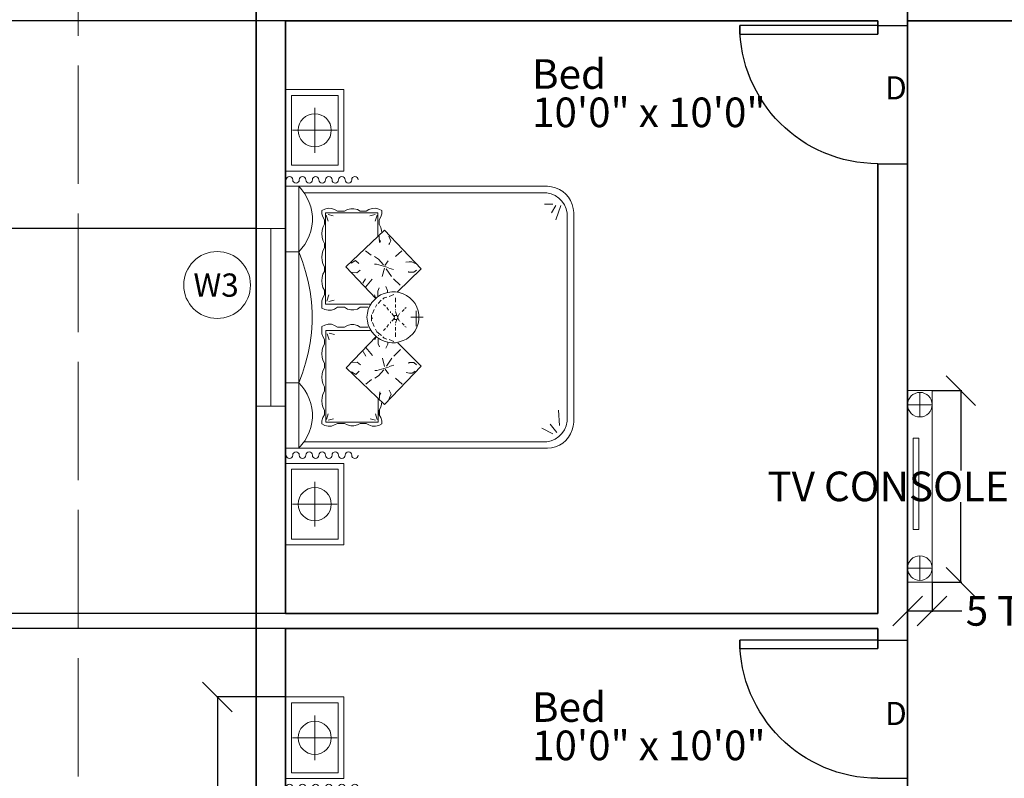
# Model space of a CAD drawing. Units: inches. Extents: x -1198 to -69, y -512 to 437.
# Tile 4 of 50: x -1067 to -867, y 5 to 158. Entities that reach past the tile are written whole.
import ezdxf

# ---------------------------------------------------------------- set-up
doc = ezdxf.new("R2010")
doc.units = ezdxf.units.IN
doc.header["$MEASUREMENT"] = 0
doc.linetypes.add('ACAD_ISO02W100', pattern=[15, 12, -3])
for name, color, linetype, lineweight in [('A-ANNO-DIMS', 2, 'Continuous', 18), ('A-ANNO-SYMB', 7, 'Continuous', 18), ('A-AREA-IDEN', 7, 'Continuous', 18), ('A-EQPM', 60, 'Continuous', 18), ('A-FURN', 60, 'Continuous', 18), ('A-WALL', 7, 'Continuous', 35), ('C-PROP', 141, 'ACAD_ISO02W100', 18), ('Doors', 140, 'Continuous', 25), ('ds_furniture_Pen_No__7', 7, 'Continuous', 18), ('windows', 160, 'Continuous', 18)]:
    doc.layers.add(name, color=color, linetype=linetype, lineweight=lineweight)
doc.styles.get("Standard").update_dxf_attribs({"font": 'arial.ttf'})
doc.dimstyles.get("Standard").update_dxf_attribs({"dimtxt": 6, "dimasz": 6, "dimexe": 0.18, "dimexo": 0.0625, "dimgap": 0.09, "dimtad": 0, "dimtih": 1, "dimtoh": 1, "dimdec": 0, "dimzin": 0, "dimdsep": 46, "dimlunit": 4, "dimtxsty": 'Standard', "dimblk": 'OBLIQUE', "dimcen": 0.09, "dimadec": 0, "dimazin": 0, "dimtfac": 1, "dimtdec": 0, "dimtofl": 0, "dimtmove": 0, "dimatfit": 3, "dimfxl": 1, "dimtolj": 1, "dimtzin": 0, "dimarcsym": 0})

# ---------------------------------------------------------------- blocks, each defined once
blk = doc.blocks.new('*U4')
for p, q in [((0, 0), (0, -6)), ((28, 0), (28, -6))]:
    blk.add_line(p, q)
blk.add_lwpolyline([(0, 0), (0, 28), (1.75, 28), (1.75, 0)], close=True)
blk.add_arc((0, 0), 28, 0, 90)
blk = doc.blocks.new('new')
at = {"layer": 'ds_furniture_Pen_No__7'}
for p, q in [((-1180, 2274.4), (-1838.2, 2274.4)), ((-1838.2, 2274.4), (-1838.2, 1804.2)), ((-1227, 2227.4), (-1791.2, 2227.4)), ((-1791.2, 2227.4), (-1791.2, 1851.2)), ((-1227, 1851.2), (-1227, 2227.4)), ((-1180, 1804.2), (-1180, 2274.4)), ((-1057.8, 158.7), (-1057.8, 2274.4)), ((-1057.8, 2274.4), (1057.8, 2274.4)), ((-1057.8, 2274.4), (1057.8, 2274.4)), ((-1057.8, 158.7), (-1057.8, 2274.4)), ((-528.9, 2274.4), (-528.9, 2168.6)), ((528.9, 2274.4), (528.9, 2168.6)), ((1057.8, 2274.4), (1057.8, 158.7)), ((1057.8, 2274.4), (1057.8, 158.7)), ((1180, 1804.2), (1180, 2274.4)), ((1180, 2274.4), (1838.2, 2274.4)), ((1227, 1851.2), (1227, 2227.4)), ((1227, 2227.4), (1791.2, 2227.4)), ((1791.2, 2227.4), (1791.2, 1851.2)), ((1838.2, 2274.4), (1838.2, 1804.2)), ((-1509.1, 2220.2), (-1509.1, 1858.4)), ((1057.8, 2168.6), (-1057.8, 2168.6)), ((-1057.8, 2168.6), (-1028.2, 2143.2)), ((-556.4, 2143.2), (-528.9, 2168.6)), ((-528.9, 2168.6), (-450.6, 2139)), ((450.6, 2139), (528.9, 2168.6)), ((528.9, 2168.6), (556.4, 2143.2)), ((1028.2, 2143.2), (1057.8, 2168.6)), ((1509.1, 2220.2), (1509.1, 1858.4)), ((-1028.2, 2143.2), (-996.5, 2119.9)), ((-1005, 165), (-1005, 2124.2)), ((-996.5, 2119.9), (-962.6, 2100.9)), ((-962.6, 2100.9), (-926.7, 2084)), ((-926.7, 2084), (-890.7, 2071.3)), ((-890.7, 2071.3), (-850.5, 2062.8)), ((-734.1, 2062.8), (-696.1, 2071.3)), ((-696.1, 2071.3), (-658, 2084)), ((-658, 2084), (-622, 2100.9)), ((-622, 2100.9), (-588.2, 2119.9)), ((-588.2, 2119.9), (-556.4, 2143.2)), ((-450.6, 2139), (-370.2, 2113.6)), ((-370.2, 2113.6), (-289.9, 2092.4)), ((-289.9, 2092.4), (-207.3, 2075.5)), ((-207.3, 2075.5), (-124.8, 2064.9)), ((124.8, 2064.9), (207.3, 2075.5)), ((207.3, 2075.5), (289.9, 2092.4)), ((289.9, 2092.4), (370.2, 2113.6)), ((370.2, 2113.6), (450.6, 2139)), ((556.4, 2143.2), (588.2, 2119.9)), ((588.2, 2119.9), (622, 2100.9)), ((622, 2100.9), (658, 2084)), ((658, 2084), (696.1, 2071.3)), ((696.1, 2071.3), (734.1, 2062.8)), ((850.5, 2062.8), (890.7, 2071.3)), ((890.7, 2071.3), (926.7, 2084)), ((926.7, 2084), (962.6, 2100.9)), ((962.6, 2100.9), (996.5, 2119.9)), ((996.5, 2119.9), (1028.2, 2143.2)), ((1005, 2124.2), (1005, 165)), ((-1690.1, 2039.3), (-1328.2, 2039.3)), ((-850.5, 2062.8), (-812.4, 2058.6)), ((-812.4, 2058.6), (-772.2, 2058.6)), ((-772.2, 2058.6), (-734.1, 2062.8)), ((-124.8, 2064.9), (-42.3, 2060.7)), ((-42.3, 2060.7), (42.3, 2060.7)), ((42.3, 2060.7), (124.8, 2064.9)), ((734.1, 2062.8), (772.2, 2058.6)), ((772.2, 2058.6), (812.4, 2058.6)), ((812.4, 2058.6), (850.5, 2062.8)), ((1690.1, 2039.3), (1328.2, 2039.3)), ((-880.1, 1931.6), (-873.8, 1959.1)), ((-878, 1904.1), (-880.1, 1931.6)), ((-873.8, 1959.1), (-861.1, 1982.4)), ((-861.1, 1982.4), (-835.7, 1982.4)), ((-846.3, 1527.5), (-846.3, 1950.7)), ((-846.3, 1950.7), (-107.9, 1950.7)), ((-835.7, 1982.4), (-810.3, 1973.9)), ((-831.5, 1929.5), (-820.9, 1887.2)), ((-825.1, 1944.3), (-778.6, 1929.5)), ((-810.3, 1973.9), (-787, 1961.2)), ((-787, 1961.2), (-751.1, 1961.2)), ((-751.1, 1961.2), (-725.7, 1973.9)), ((-725.7, 1973.9), (-700.3, 1980.3)), ((-700.3, 1980.3), (-674.9, 1982.4)), ((-674.9, 1982.4), (-647.4, 1980.3)), ((-647.4, 1980.3), (-622, 1973.9)), ((-622, 1973.9), (-596.6, 1961.2)), ((-596.6, 1961.2), (-560.7, 1961.2)), ((-560.7, 1961.2), (-535.3, 1973.9)), ((-535.3, 1973.9), (-509.9, 1980.3)), ((-509.9, 1980.3), (-484.5, 1982.4)), ((-484.5, 1982.4), (-457, 1980.3)), ((-457, 1980.3), (-431.6, 1973.9)), ((-431.6, 1973.9), (-408.3, 1961.2)), ((-408.3, 1961.2), (-370.2, 1961.2)), ((-370.2, 1961.2), (-347, 1973.9)), ((-347, 1973.9), (-321.6, 1980.3)), ((-321.6, 1980.3), (-294.1, 1982.4)), ((-294.1, 1982.4), (-266.6, 1980.3)), ((-266.6, 1980.3), (-241.2, 1973.9)), ((-241.2, 1973.9), (-217.9, 1961.2)), ((-217.9, 1961.2), (-179.8, 1961.2)), ((-133.3, 1940.1), (-181.9, 1923.2)), ((-179.8, 1961.2), (-156.6, 1973.9)), ((-156.6, 1973.9), (-133.3, 1982.4)), ((-129.1, 1923.2), (-139.6, 1880.9)), ((-133.3, 1982.4), (-105.8, 1982.4)), ((-107.9, 1950.7), (-107.9, 1591)), ((-105.8, 1982.4), (-74, 1982.4)), ((-74, 1982.4), (-63.5, 1959.1)), ((-63.5, 1959.1), (-57.1, 1931.6)), ((-57.1, 1931.6), (-57.1, 1904.1)), ((63.5, 1959.1), (57.1, 1931.6)), ((57.1, 1931.6), (57.1, 1904.1)), ((74, 1982.4), (63.5, 1959.1)), ((105.8, 1982.4), (74, 1982.4)), ((133.3, 1982.4), (105.8, 1982.4)), ((844.2, 1952.8), (105.8, 1952.8)), ((105.8, 1952.8), (105.8, 1593.1)), ((126.9, 1925.3), (137.5, 1883)), ((131.2, 1942.2), (179.8, 1925.3)), ((156.6, 1973.9), (133.3, 1982.4)), ((179.8, 1961.2), (156.6, 1973.9)), ((217.9, 1961.2), (179.8, 1961.2)), ((241.2, 1973.9), (217.9, 1961.2)), ((266.6, 1980.3), (241.2, 1973.9)), ((294.1, 1982.4), (266.6, 1980.3)), ((321.6, 1980.3), (294.1, 1982.4)), ((347, 1973.9), (321.6, 1980.3)), ((370.2, 1961.2), (347, 1973.9)), ((408.3, 1961.2), (370.2, 1961.2)), ((431.6, 1973.9), (408.3, 1961.2)), ((457, 1980.3), (431.6, 1973.9)), ((484.5, 1982.4), (457, 1980.3)), ((509.9, 1980.3), (484.5, 1982.4)), ((535.3, 1973.9), (509.9, 1980.3)), ((560.7, 1961.2), (535.3, 1973.9)), ((596.6, 1961.2), (560.7, 1961.2)), ((622, 1973.9), (596.6, 1961.2)), ((647.4, 1980.3), (622, 1973.9)), ((674.9, 1982.4), (647.4, 1980.3)), ((700.3, 1980.3), (674.9, 1982.4)), ((725.7, 1973.9), (700.3, 1980.3)), ((751.1, 1961.2), (725.7, 1973.9)), ((787, 1961.2), (751.1, 1961.2)), ((823, 1946.4), (776.5, 1931.6)), ((810.3, 1973.9), (787, 1961.2)), ((835.7, 1982.4), (810.3, 1973.9)), ((829.4, 1931.6), (818.8, 1889.3)), ((861.1, 1982.4), (835.7, 1982.4)), ((844.2, 1529.6), (844.2, 1952.8)), ((873.8, 1959.1), (861.1, 1982.4)), ((880.1, 1931.6), (873.8, 1959.1)), ((878, 1904.1), (880.1, 1931.6)), ((-1791.2, 1851.2), (-1227, 1851.2)), ((-869.6, 1878.7), (-878, 1904.1)), ((-856.9, 1855.5), (-869.6, 1878.7)), ((-856.9, 1798.3), (-856.9, 1855.5)), ((-65.6, 1878.7), (-80.4, 1855.5)), ((-80.4, 1855.5), (-80.4, 1798.3)), ((-57.1, 1904.1), (-65.6, 1878.7)), ((57.1, 1904.1), (65.6, 1878.7)), ((65.6, 1878.7), (80.4, 1855.5)), ((80.4, 1855.5), (80.4, 1798.3)), ((856.9, 1855.5), (869.6, 1878.7)), ((856.9, 1798.3), (856.9, 1855.5)), ((869.6, 1878.7), (878, 1904.1)), ((1791.2, 1851.2), (1227, 1851.2)), ((-1838.2, 1804.2), (-1180, 1804.2)), ((-875.9, 1747.6), (-869.6, 1775.1)), ((-869.6, 1775.1), (-856.9, 1798.3)), ((-704.5, 1474.6), (-408.3, 1785.6)), ((-408.3, 1785.6), (-154.4, 1544.5)), ((-366, 1749.7), (-361.8, 1696.8)), ((-80.4, 1798.3), (-65.6, 1775.1)), ((-65.6, 1775.1), (-59.2, 1747.6)), ((65.6, 1775.1), (59.2, 1747.6)), ((80.4, 1798.3), (65.6, 1775.1)), ((406.2, 1787.8), (152.3, 1546.6)), ((363.9, 1751.8), (359.7, 1698.9)), ((702.4, 1476.8), (406.2, 1787.8)), ((869.6, 1775.1), (856.9, 1798.3)), ((875.9, 1747.6), (869.6, 1775.1)), ((1838.2, 1804.2), (1180, 1804.2)), ((-875.9, 1722.2), (-875.9, 1747.6)), ((-869.6, 1694.7), (-875.9, 1722.2)), ((-856.9, 1671.4), (-869.6, 1694.7)), ((-856.9, 1624.9), (-856.9, 1671.4)), ((-440.1, 1743.3), (-461.2, 1707.4)), ((-461.2, 1707.4), (-435.8, 1679.9)), ((-361.8, 1696.8), (-382.9, 1669.3)), ((-65.6, 1694.7), (-80.4, 1671.4)), ((-80.4, 1671.4), (-80.4, 1607.9)), ((-59.2, 1722.2), (-65.6, 1694.7)), ((-59.2, 1747.6), (-59.2, 1722.2)), ((59.2, 1747.6), (59.2, 1722.2)), ((59.2, 1722.2), (65.6, 1694.7)), ((65.6, 1694.7), (80.4, 1671.4)), ((80.4, 1671.4), (80.4, 1607.9)), ((359.7, 1698.9), (380.8, 1671.4)), ((459.1, 1709.5), (433.7, 1682)), ((437.9, 1745.4), (459.1, 1709.5)), ((856.9, 1671.4), (869.6, 1694.7)), ((856.9, 1624.9), (856.9, 1671.4)), ((869.6, 1694.7), (875.9, 1722.2)), ((875.9, 1722.2), (875.9, 1747.6)), ((-878, 1576.2), (-869.6, 1601.6)), ((-869.6, 1601.6), (-856.9, 1624.9)), ((-831.5, 1548.7), (-820.9, 1591)), ((-539.5, 1627), (-503.5, 1580.4)), ((-277.2, 1648.1), (-313.1, 1627)), ((-245.4, 1627), (-308.9, 1574.1)), ((-118.5, 1578.3), (-91, 1595.2)), ((-91, 1595.2), (-61.4, 1607.9)), ((-61.4, 1607.9), (-31.7, 1614.3)), ((-31.7, 1614.3), (0, 1618.5)), ((0, 1618.5), (31.7, 1614.3)), ((31.7, 1614.3), (61.4, 1607.9)), ((61.4, 1607.9), (91, 1595.2)), ((91, 1595.2), (118.5, 1578.3)), ((243.3, 1629.1), (306.8, 1576.2)), ((275, 1650.2), (311, 1629.1)), ((537.4, 1629.1), (501.4, 1582.5)), ((829.4, 1550.8), (818.8, 1593.1)), ((869.6, 1601.6), (856.9, 1624.9)), ((878, 1576.2), (869.6, 1601.6)), ((-880.1, 1548.7), (-878, 1576.2)), ((-873.8, 1521.2), (-880.1, 1548.7)), ((-861.1, 1497.9), (-873.8, 1521.2)), ((-651.6, 1527.5), (-846.3, 1527.5)), ((-825.1, 1533.9), (-778.6, 1548.7)), ((-787, 1519.1), (-810.3, 1506.4)), ((-772.2, 1517), (-789.2, 1517)), ((-751.1, 1519.1), (-787, 1519.1)), ((-761.7, 1517), (-772.2, 1517)), ((-751.1, 1517), (-761.7, 1517)), ((-725.7, 1506.4), (-751.1, 1519.1)), ((-655.9, 1517), (-634.7, 1517)), ((-634.7, 1517), (-613.6, 1506.4)), ((-613.6, 1506.4), (-630.5, 1517)), ((-630.5, 1517), (-603, 1512.7)), ((-471.8, 1523.3), (-493, 1555)), ((-425.3, 1481), (-471.8, 1523.3)), ((-429.5, 1538.1), (-429.5, 1555)), ((-414.7, 1481), (-429.5, 1538.1)), ((-213.7, 1527.5), (-239.1, 1517)), ((-175.6, 1527.5), (-213.7, 1527.5)), ((-181.9, 1555), (-154.4, 1544.5)), ((-179.8, 1508.5), (-162.9, 1533.9)), ((-175.6, 1527.5), (-171.4, 1523.3)), ((-162.9, 1533.9), (-141.8, 1557.2)), ((-116.4, 1538.1), (-148.1, 1500)), ((-148.1, 1527.5), (-143.9, 1521.2)), ((-141.8, 1557.2), (-118.5, 1578.3)), ((-116.4, 1538.1), (-95.2, 1548.7)), ((-42.3, 1574.1), (-74, 1559.3)), ((-31.7, 1580.4), (-2.1, 1580.4)), ((19, 1580.4), (-10.6, 1580.4)), ((-6.3, 1584.7), (-6.3, 1569.8)), ((-6.3, 1584.7), (-6.3, 1569.8)), ((29.6, 1574.1), (61.4, 1559.3)), ((103.7, 1538.1), (82.5, 1548.7)), ((112.1, 1527.5), (137.5, 1502.1)), ((118.5, 1578.3), (141.8, 1557.2)), ((141.8, 1557.2), (162.9, 1533.9)), ((179.8, 1557.2), (152.3, 1546.6)), ((162.9, 1533.9), (179.8, 1508.5)), ((173.5, 1529.6), (169.3, 1525.4)), ((173.5, 1529.6), (211.6, 1529.6)), ((211.6, 1529.6), (237, 1519.1)), ((412.6, 1483.1), (427.4, 1540.2)), ((423.1, 1483.1), (469.7, 1525.4)), ((427.4, 1540.2), (427.4, 1557.2)), ((469.7, 1525.4), (490.8, 1557.2)), ((628.4, 1519.1), (600.9, 1514.8)), ((632.6, 1519.1), (611.4, 1508.5)), ((611.4, 1508.5), (628.4, 1519.1)), ((653.7, 1519.1), (632.6, 1519.1)), ((649.5, 1529.6), (844.2, 1529.6)), ((725.7, 1506.4), (751.1, 1519.1)), ((749, 1519.1), (759.5, 1519.1)), ((751.1, 1519.1), (787, 1519.1)), ((759.5, 1519.1), (770.1, 1519.1)), ((770.1, 1519.1), (787, 1519.1)), ((823, 1536), (776.5, 1550.8)), ((787, 1519.1), (810.3, 1506.4)), ((861.1, 1497.9), (873.8, 1521.2)), ((873.8, 1521.2), (880.1, 1548.7)), ((880.1, 1548.7), (878, 1576.2)), ((-835.7, 1497.9), (-861.1, 1497.9)), ((-810.3, 1506.4), (-835.7, 1497.9)), ((-700.3, 1500), (-725.7, 1506.4)), ((-393.5, 1178.4), (-704.5, 1474.6)), ((-683.4, 1497.9), (-700.3, 1500)), ((-655.9, 1438.7), (-619.9, 1421.7)), ((-619.9, 1421.7), (-598.7, 1432.3)), ((-598.7, 1432.3), (-588.2, 1438.7)), ((-457, 1442.9), (-418.9, 1470.4)), ((-404.1, 1442.9), (-414.7, 1481)), ((-397.8, 1474.6), (-330, 1491.6)), ((-397.8, 1438.7), (-387.2, 1400.6)), ((-393.5, 1459.8), (-330, 1417.5)), ((-217.9, 1449.3), (-249.7, 1464.1)), ((-217.9, 1449.3), (-203.1, 1449.3)), ((-205.2, 1417.5), (-201, 1449.3)), ((-201, 1449.3), (-192.5, 1478.9)), ((-196.8, 1400.6), (-179.8, 1438.7)), ((-192.5, 1478.9), (-179.8, 1508.5)), ((-169.3, 1478.9), (-175.6, 1457.7)), ((-169.3, 1478.9), (-158.7, 1489.4)), ((-91, 1468.3), (-105.8, 1485.2)), ((-59.2, 1442.9), (-80.4, 1457.7)), ((57.1, 1442.9), (78.3, 1457.7)), ((88.9, 1468.3), (103.7, 1485.2)), ((156.6, 1478.9), (146, 1489.4)), ((156.6, 1478.9), (162.9, 1457.7)), ((184.1, 1400.6), (167.1, 1438.7)), ((179.8, 1508.5), (192.5, 1478.9)), ((192.5, 1478.9), (201, 1449.3)), ((215.8, 1451.4), (201, 1451.4)), ((201, 1449.3), (205.2, 1417.5)), ((215.8, 1451.4), (247.5, 1466.2)), ((395.6, 1476.8), (327.9, 1493.7)), ((391.4, 1461.9), (327.9, 1419.6)), ((395.6, 1440.8), (385.1, 1402.7)), ((391.4, 1180.6), (702.4, 1476.8)), ((402, 1445), (412.6, 1483.1)), ((454.9, 1445), (416.8, 1472.5)), ((596.6, 1434.4), (586, 1440.8)), ((617.8, 1423.9), (596.6, 1434.4)), ((653.7, 1440.8), (617.8, 1423.9)), ((683.4, 1497.9), (700.3, 1500)), ((700.3, 1500), (725.7, 1506.4)), ((810.3, 1506.4), (835.7, 1497.9)), ((835.7, 1497.9), (861.1, 1497.9)), ((-539.5, 1332.9), (-493, 1385.8)), ((-393.5, 1178.4), (-207.3, 1368.9)), ((-260.2, 1347.7), (-313.1, 1400.6)), ((-205.2, 1385.8), (-205.2, 1417.5)), ((-198.9, 1356.2), (-205.2, 1385.8)), ((-188.3, 1324.4), (-198.9, 1356.2)), ((-122.7, 1385.8), (-158.7, 1385.8)), ((-80.4, 1385.8), (-105.8, 1385.8)), ((-59.2, 1385.8), (-63.5, 1385.8)), ((-38.1, 1428.1), (-48.7, 1428.1)), ((-16.9, 1375.2), (-48.7, 1385.8)), ((-6.3, 1396.4), (-31.7, 1417.5)), ((-6.3, 1368.9), (-31.7, 1354)), ((-16.9, 1385.8), (-16.9, 1396.4)), ((-16.9, 1396.4), (-6.3, 1396.4)), ((-16.9, 1375.2), (-16.9, 1385.8)), ((-6.3, 1368.9), (-16.9, 1375.2)), ((-6.3, 1396.4), (-2.1, 1398.5)), ((-6.3, 1368.9), (-2.1, 1368.9)), ((4.2, 1396.4), (-2.1, 1398.5)), ((4.2, 1368.9), (-2.1, 1368.9)), ((4.2, 1396.4), (29.6, 1417.5)), ((14.8, 1396.4), (4.2, 1396.4)), ((4.2, 1368.9), (14.8, 1375.2)), ((4.2, 1368.9), (29.6, 1354)), ((14.8, 1385.8), (14.8, 1396.4)), ((14.8, 1375.2), (14.8, 1385.8)), ((14.8, 1375.2), (46.5, 1385.8)), ((36, 1428.1), (46.5, 1428.1)), ((57.1, 1385.8), (61.4, 1385.8)), ((78.3, 1385.8), (103.7, 1385.8)), ((120.6, 1385.8), (156.6, 1385.8)), ((198.9, 1356.2), (188.3, 1324.4)), ((205.2, 1385.8), (198.9, 1356.2)), ((205.2, 1417.5), (205.2, 1385.8)), ((391.4, 1180.6), (205.2, 1371)), ((258.1, 1349.8), (311, 1402.7)), ((537.4, 1335), (490.8, 1387.9)), ((-450.6, 1273.6), (-446.4, 1301.2)), ((-450.6, 1252.5), (-450.6, 1273.6)), ((-366, 1280), (-372.4, 1280)), ((-366, 1237.7), (-366, 1280)), ((-175.6, 1296.9), (-188.3, 1324.4)), ((-156.6, 1271.5), (-175.6, 1296.9)), ((-74, 1311.7), (-80.4, 1301.2)), ((-48.7, 1332.9), (-63.5, 1316)), ((-38.1, 1343.5), (-38, 1343.5)), ((36, 1343.5), (36, 1343.5)), ((46.5, 1332.9), (61.4, 1316)), ((71.9, 1311.7), (78.3, 1301.2)), ((175.6, 1296.9), (156.6, 1271.5)), ((188.3, 1324.4), (175.6, 1296.9)), ((363.9, 1239.8), (363.9, 1282.1)), ((363.9, 1282.1), (370.2, 1282.1)), ((448.5, 1275.8), (444.3, 1303.3)), ((448.5, 1254.6), (448.5, 1275.8)), ((-435.8, 1227.1), (-450.6, 1252.5)), ((-382.9, 1216.5), (-366, 1237.7)), ((-133.3, 1248.3), (-156.6, 1271.5)), ((-110, 1229.2), (-133.3, 1248.3)), ((-80.4, 1214.4), (-110, 1229.2)), ((-50.8, 1203.8), (-80.4, 1214.4)), ((52.9, 1220.8), (-71.9, 1220.8)), ((-21.2, 1197.5), (-50.8, 1203.8)), ((0, 1197.5), (-21.2, 1197.5)), ((0, 1163.6), (0, 1263.1)), ((21.2, 1197.5), (0, 1197.5)), ((50.8, 1203.8), (21.2, 1197.5)), ((80.4, 1214.4), (50.8, 1203.8)), ((110, 1229.2), (80.4, 1214.4)), ((133.3, 1248.3), (110, 1229.2)), ((156.6, 1271.5), (133.3, 1248.3)), ((380.8, 1218.6), (363.9, 1239.8)), ((433.7, 1229.2), (448.5, 1254.6)), ((-996.5, 129.1), (-1005, 165)), ((-941.5, 116.4), (-894.9, 205.2)), ((914, 116.4), (914, 184.1)), ((1005, 165), (996.5, 129.1)), ((-1053.6, 126.9), (-1057.8, 158.7)), ((-1053.6, 126.9), (-1057.8, 158.7)), ((-1045.2, 95.2), (-1053.6, 126.9)), ((-1045.2, 95.2), (-1053.6, 126.9)), ((-1032.5, 63.5), (-1045.2, 95.2)), ((-1032.5, 63.5), (-1045.2, 95.2)), ((-983.8, 97.3), (-996.5, 129.1)), ((-962.6, 67.7), (-983.8, 97.3)), ((-930.9, 84.6), (-863.2, 137.5)), ((903.4, 52.9), (787, 91)), ((903.4, 91), (844.2, 126.9)), ((983.8, 97.3), (962.6, 67.7)), ((996.5, 129.1), (983.8, 97.3)), ((1045.2, 95.2), (1032.5, 63.5)), ((1045.2, 95.2), (1032.5, 63.5)), ((1053.6, 126.9), (1045.2, 95.2)), ((1053.6, 126.9), (1045.2, 95.2)), ((1057.8, 158.7), (1053.6, 126.9)), ((1057.8, 158.7), (1053.6, 126.9)), ((-1015.5, 36), (-1032.5, 63.5)), ((-1015.5, 36), (-1032.5, 63.5)), ((-994.4, 10.6), (-1015.5, 36)), ((-994.4, 10.6), (-1015.5, 36)), ((-969, -10.6), (-994.4, 10.6)), ((-969, -10.6), (-994.4, 10.6)), ((-937.3, 42.3), (-962.6, 67.7)), ((-907.6, 21.2), (-937.3, 42.3)), ((-875.9, 8.5), (-907.6, 21.2)), ((-839.9, 0), (-875.9, 8.5)), ((-873.8, 63.5), (-751.1, 69.8)), ((839.9, 0), (-839.9, 0)), ((875.9, 8.5), (839.9, 0)), ((907.6, 21.2), (875.9, 8.5)), ((937.3, 42.3), (907.6, 21.2)), ((962.6, 67.7), (937.3, 42.3)), ((994.4, 10.6), (969, -10.6)), ((994.4, 10.6), (969, -10.6)), ((1015.5, 36), (994.4, 10.6)), ((1015.5, 36), (994.4, 10.6)), ((1032.5, 63.5), (1015.5, 36)), ((1032.5, 63.5), (1015.5, 36)), ((-941.5, -27.5), (-969, -10.6)), ((-941.5, -27.5), (-969, -10.6)), ((-909.7, -40.2), (-941.5, -27.5)), ((-909.7, -40.2), (-941.5, -27.5)), ((-878, -48.7), (-909.7, -40.2)), ((-878, -48.7), (-909.7, -40.2)), ((-846.3, -52.9), (-878, -48.7)), ((-846.3, -52.9), (-878, -48.7)), ((846.3, -52.9), (-846.3, -52.9)), ((846.3, -52.9), (-846.3, -52.9)), ((878, -48.7), (846.3, -52.9)), ((878, -48.7), (846.3, -52.9)), ((909.7, -40.2), (878, -48.7)), ((909.7, -40.2), (878, -48.7)), ((941.5, -27.5), (909.7, -40.2)), ((941.5, -27.5), (909.7, -40.2)), ((969, -10.6), (941.5, -27.5)), ((969, -10.6), (941.5, -27.5))]:
    blk.add_line(p, q, dxfattribs=at)
for centre in [(-1509.1, 2039.3), (1509.1, 2039.3)]:
    blk.add_circle(centre, 133.9, dxfattribs=at)
for centre, start, end in [((-1112.8, 2243.5), 90, 270), ((1108.7, 2243.5), 270, 90), ((-1112.8, 2137.7), 90, 270), ((-1112.8, 2190.6), 270, 90), ((1108.7, 2190.6), 90, 270), ((1108.7, 2137.7), 270, 90), ((-1112.8, 2084.8), 270, 90), ((-1112.8, 2084.8), 270, 90), ((1108.7, 2084.8), 90, 270), ((1108.7, 2084.8), 90, 270), ((-1112.8, 2031.9), 90, 270), ((-1112.8, 1979), 270, 90), ((1108.7, 1979), 90, 270), ((1108.7, 2031.9), 270, 90), ((-1112.8, 1926.1), 90, 270), ((1108.7, 1926.1), 270, 90), ((-1112.8, 1820.3), 90, 270), ((-1112.8, 1873.2), 270, 90), ((1108.7, 1873.2), 90, 270), ((1108.7, 1820.3), 270, 90), ((-1112.8, 1767.4), 270, 90), ((1108.7, 1767.4), 90, 270), ((-1112.8, 1714.6), 90, 270), ((1108.7, 1714.6), 270, 90)]:
    blk.add_arc(centre, 26.4, start, end, dxfattribs=at)
blk = doc.blocks.new('WIN-W3-36')
at = {"ltscale": 10}
for p, q in [((0, 6), (0, 0)), ((36, 6), (36, 0)), ((0, 3), (36, 3))]:
    blk.add_line(p, q, dxfattribs=at)
blk = doc.blocks.new('TV-CONSOLE')
at = {"ltscale": 10}
for p, q in [((2.49, 33.45), (2.49, 38.43)), ((4.97, 35.94), (0, 35.94)), ((2.49, 5.34), (2.49, 0.37)), ((4.97, 2.85), (0, 2.85))]:
    blk.add_line(p, q, dxfattribs=at)
for points in [[(4.97, 38.79), (0, 38.79), (0, 0), (4.97, 0)], [(2.27, 29.19), (1.16, 29.19), (1.16, 10.69), (2.27, 10.69)]]:
    blk.add_lwpolyline(points, close=True, dxfattribs=at)
for centre in [(2.49, 35.94), (2.49, 2.85)]:
    blk.add_circle(centre, 2.49, dxfattribs=at)
blk = doc.blocks.new('TAG-W3')
at = {"ltscale": 10}
blk.add_circle((0, 0), 6.77, dxfattribs=at)
blk.add_text('W3', height=4.7, dxfattribs=at).set_placement((-4.79, -2.36))
blk = doc.blocks.new('_Oblique')
at = {"color": 0, "linetype": 'ByBlock', "lineweight": -2}
blk.add_line((-0.5, -0.5), (0.5, 0.5), dxfattribs=at)
blk = doc.blocks.new('*D38')
at = {"layer": 'A-ANNO-DIMS', "color": 0, "lineweight": -2, "ltscale": 10, "transparency": 16777216}
for p, q in [((-1012.81, 21.34), (-1026.76, 21.34)), ((-1026.58, 21.34), (-1026.58, -21.58)), ((-1026.58, -70.88), (-1026.58, -27.97)), ((-1012.81, -70.88), (-1026.76, -70.88))]:
    blk.add_line(p, q, dxfattribs=at)
at = {"layer": 'DEFPOINTS', "color": 0, "ltscale": 10, "transparency": 16777216}
for p in [(-1026.58, 21.34), (-1012.75, 21.34), (-1012.75, -70.88)]:
    blk.add_point(p, dxfattribs=at)
at = {"layer": 'A-ANNO-DIMS', "color": 0, "lineweight": -2, "ltscale": 10, "transparency": 16777216, "xscale": 6, "yscale": 6, "zscale": 6}
for p, rotation in [((-1026.58, 21.34), 90), ((-1026.58, -70.88), 270)]:
    blk.add_blockref('_Oblique', p, dxfattribs=dict(at, rotation=rotation))
at = {"layer": 'A-ANNO-DIMS', "color": 0, "ltscale": 10, "transparency": 16777216, "insert": (-1026.58, -24.77), "char_height": 6, "attachment_point": 5}
blk.add_mtext('\\A1;BED GROUP 92 TYP.', dxfattribs=at)
blk = doc.blocks.new('*D58')
at = {"layer": 'A-ANNO-DIMS', "color": 0, "lineweight": -2, "ltscale": 10, "transparency": 16777216}
for p, q in [((-881.72, 83.38), (-875.78, 83.38)), ((-875.96, 83.38), (-875.96, 67.18)), ((-875.96, 44.58), (-875.96, 60.78)), ((-881.72, 44.58), (-875.78, 44.58))]:
    blk.add_line(p, q, dxfattribs=at)
at = {"layer": 'DEFPOINTS', "color": 0, "ltscale": 10, "transparency": 16777216}
for p in [(-881.78, 83.38), (-875.96, 83.38), (-881.78, 44.58)]:
    blk.add_point(p, dxfattribs=at)
at = {"layer": 'A-ANNO-DIMS', "color": 0, "lineweight": -2, "ltscale": 10, "transparency": 16777216, "xscale": 6, "yscale": 6, "zscale": 6}
for p, rotation in [((-875.96, 83.38), 90), ((-875.96, 44.58), 270)]:
    blk.add_blockref('_Oblique', p, dxfattribs=dict(at, rotation=rotation))
at = {"layer": 'A-ANNO-DIMS', "color": 0, "ltscale": 10, "transparency": 16777216, "insert": (-875.96, 63.98), "char_height": 6, "attachment_point": 5}
blk.add_mtext('\\A1;TV CONSOLE 39 TYP.', dxfattribs=at)
blk = doc.blocks.new('*D59')
at = {"layer": 'A-ANNO-DIMS', "color": 0, "lineweight": -2, "ltscale": 10, "transparency": 16777216}
for p, q in [((-886.75, 44.52), (-886.75, 38.59)), ((-881.78, 44.52), (-881.78, 38.59)), ((-886.75, 38.77), (-881.78, 38.77)), ((-881.78, 38.77), (-875.78, 38.77))]:
    blk.add_line(p, q, dxfattribs=at)
at = {"layer": 'DEFPOINTS', "color": 0, "ltscale": 10, "transparency": 16777216}
for p in [(-886.75, 44.58), (-881.78, 44.58), (-881.78, 38.77)]:
    blk.add_point(p, dxfattribs=at)
at = {"layer": 'A-ANNO-DIMS', "color": 0, "lineweight": -2, "ltscale": 10, "transparency": 16777216, "xscale": 6, "yscale": 6, "zscale": 6, "rotation": 180}
blk.add_blockref('_Oblique', (-886.75, 38.77), dxfattribs=at)
at = {"layer": 'A-ANNO-DIMS', "color": 0, "lineweight": -2, "ltscale": 10, "transparency": 16777216, "xscale": 6, "yscale": 6, "zscale": 6}
blk.add_blockref('_Oblique', (-881.78, 38.77), dxfattribs=at)
at = {"layer": 'A-ANNO-DIMS', "color": 0, "ltscale": 10, "transparency": 16777216, "insert": (-863.42, 38.77), "char_height": 6, "attachment_point": 5}
blk.add_mtext('\\A1;5 TYP.', dxfattribs=at)
blk = doc.blocks.new('*D61')
at = {"layer": 'A-ANNO-DIMS', "color": 0, "lineweight": -2, "ltscale": 10, "transparency": 16777216}
for p, q in [((-1054.81, 299.23), (-1188.2, 299.23)), ((-1188.02, 299.23), (-1188.02, 20.38)), ((-1188.02, -264.77), (-1188.02, 14.07)), ((-1054.81, -264.77), (-1188.2, -264.77))]:
    blk.add_line(p, q, dxfattribs=at)
at = {"layer": 'DEFPOINTS', "color": 0, "ltscale": 10, "transparency": 16777216}
for p in [(-1054.75, 299.23), (-1188.02, -264.77), (-1054.75, -264.77)]:
    blk.add_point(p, dxfattribs=at)
at = {"layer": 'A-ANNO-DIMS', "color": 0, "lineweight": -2, "ltscale": 10, "transparency": 16777216, "xscale": 6, "yscale": 6, "zscale": 6}
for p, rotation in [((-1188.02, 299.23), 90), ((-1188.02, -264.77), 270)]:
    blk.add_blockref('_Oblique', p, dxfattribs=dict(at, rotation=rotation))
at = {"layer": 'A-ANNO-DIMS', "color": 0, "ltscale": 10, "transparency": 16777216, "insert": (-1188.02, 17.23), "char_height": 6, "attachment_point": 5}
blk.add_mtext('\\A1;564', dxfattribs=at)
blk = doc.blocks.new('*D74')
at = {"layer": 'A-ANNO-DIMS', "color": 0, "lineweight": -2, "ltscale": 10, "transparency": 16777216}
for p, q in [((-1012.81, 38.23), (-1188.2, 38.23)), ((-1188.02, 38.23), (-1188.02, 35.23)), ((-1012.81, 35.23), (-1188.2, 35.23)), ((-1188.02, 35.23), (-1188.02, 29.23)), ((-1188.02, 29.23), (-1194.02, 29.23))]:
    blk.add_line(p, q, dxfattribs=at)
at = {"layer": 'DEFPOINTS', "color": 0, "ltscale": 10, "transparency": 16777216}
for p in [(-1012.75, 38.23), (-1188.02, 35.23), (-1012.75, 35.23)]:
    blk.add_point(p, dxfattribs=at)
at = {"layer": 'A-ANNO-DIMS', "color": 0, "lineweight": -2, "ltscale": 10, "transparency": 16777216, "xscale": 6, "yscale": 6, "zscale": 6}
for p, rotation in [((-1188.02, 38.23), 90), ((-1188.02, 35.23), 270)]:
    blk.add_blockref('_Oblique', p, dxfattribs=dict(at, rotation=rotation))
at = {"layer": 'A-ANNO-DIMS', "color": 0, "ltscale": 10, "transparency": 16777216, "insert": (-1196.08, 29.23), "char_height": 6, "attachment_point": 5}
blk.add_mtext('\\A1;3', dxfattribs=at)
blk = doc.blocks.new('*D80')
at = {"layer": 'A-ANNO-DIMS', "color": 0, "lineweight": -2, "ltscale": 10, "transparency": 16777216}
for p, q in [((-1012.81, 158.23), (-1188.2, 158.23)), ((-1188.02, 158.23), (-1188.02, 140.33)), ((-1188.02, 116.23), (-1188.02, 134.13)), ((-1018.81, 116.23), (-1188.2, 116.23))]:
    blk.add_line(p, q, dxfattribs=at)
at = {"layer": 'DEFPOINTS', "color": 0, "ltscale": 10, "transparency": 16777216}
for p in [(-1188.02, 158.23), (-1012.75, 158.23), (-1018.75, 116.23)]:
    blk.add_point(p, dxfattribs=at)
at = {"layer": 'A-ANNO-DIMS', "color": 0, "lineweight": -2, "ltscale": 10, "transparency": 16777216, "xscale": 6, "yscale": 6, "zscale": 6}
for p, rotation in [((-1188.02, 158.23), 90), ((-1188.02, 116.23), 270)]:
    blk.add_blockref('_Oblique', p, dxfattribs=dict(at, rotation=rotation))
at = {"layer": 'A-ANNO-DIMS', "color": 0, "ltscale": 10, "transparency": 16777216, "insert": (-1188.02, 137.23), "char_height": 6, "attachment_point": 5}
blk.add_mtext('\\A1;42', dxfattribs=at)

msp = doc.modelspace()

# ---------------------------------------------------------------- linework, layer by layer
at = {"layer": 'A-WALL', "ltscale": 10}
for p, q in [((-1018.7509, 263.2277), (-1018.7509, -228.7723)), ((-886.7509, 161.2277), (-886.7509, 35.2277)), ((-892.7509, 158.2277), (-1012.7509, 158.2277)), ((-1012.7509, 158.2277), (-1012.7509, 38.2277)), ((-892.7509, 158.2277), (-892.7509, 155.5722)), ((-697.7509, 158.2277), (-886.7509, 158.2277)), ((-892.7509, 129.3222), (-892.7509, 38.2277)), ((-892.7509, 38.2277), (-1012.7509, 38.2277)), ((-892.7509, 35.2277), (-1012.7509, 35.2277)), ((-1012.7509, 35.2277), (-1012.7509, -84.7723)), ((-892.7509, 35.2277), (-892.7509, 31.124)), ((-886.7509, 35.2277), (-886.7509, -38.2723))]:
    msp.add_line(p, q, dxfattribs=at)
at = {"layer": 'C-PROP', "ltscale": 2}
msp.add_lwpolyline([(-1054.7509, 299.2277), (-334.7509, 299.2277), (-334.7509, -264.7723), (-1054.7509, -264.7723)], close=True, dxfattribs=at)

# ---------------------------------------------------------------- block references
at = {"layer": 'A-ANNO-SYMB'}
msp.add_blockref('TAG-W3', (-1026.6373, 104.7498), dxfattribs=at)
at = {"layer": 'A-EQPM'}
msp.add_blockref('TV-CONSOLE', (-886.751, 44.584), dxfattribs=at)
at = {"layer": 'A-FURN', "xscale": 0.0250833463801972, "yscale": 0.0250833463801972, "zscale": 0.0250833463801972, "rotation": 90}
for p in [(-955.702, 98.2277), (-955.702, -24.7723)]:
    msp.add_blockref('new', p, dxfattribs=at)
at = {"layer": 'Doors', "xscale": -1, "rotation": 90}
for p in [(-892.7509, 157.3222), (-892.7509, 32.874)]:
    msp.add_blockref('*U4', p, dxfattribs=at)
at = {"layer": 'windows', "rotation": 89.99999999999966}
msp.add_blockref('WIN-W3-36', (-1012.7512, 80.228), dxfattribs=at)

# ---------------------------------------------------------------- texts
at = {"layer": 'A-ANNO-SYMB', "ltscale": 10}
for p in [(-891.3184, 142.3277), (-891.3184, 15.6475)]:
    msp.add_text('D', height=4.6996, dxfattribs=at).set_placement(p)
at = {"layer": 'A-AREA-IDEN', "ltscale": 10, "char_height": 6, "attachment_point": 1}
for s, insert in [('Bed', (-962.8292, 150.4825)), ('10\'0" x 10\'0"', (-962.8292, 142.7185)), ('Bed', (-962.8292, 22.3036)), ('10\'0" x 10\'0"', (-962.8292, 14.5396))]:
    msp.add_mtext_dynamic_manual_height_columns(s, width=57.976527, gutter_width=30, heights=[0], dxfattribs=dict(at, insert=insert))

# ---------------------------------------------------------------- dimensions: what is measured, and where the dimension line sits
at = {"layer": 'A-ANNO-DIMS', "ltscale": 10}
for base, p1, p2, picture, middle in [((-1188.0248, -264.7723), (-1054.7509, 299.2277), (-1054.7509, -264.7723), '*D61', (-1188.0248, 17.2277)), ((-1188.0248, 158.2277), (-1018.7509, 116.2277), (-1012.7509, 158.2277), '*D80', (-1188.0248, 137.2277)), ((-1188.0248, 35.2277), (-1012.7509, 38.2277), (-1012.7509, 35.2277), '*D74', (-1196.0793, 29.2277))]:
    dim = msp.add_linear_dim(base=base, p1=p1, p2=p2, angle=90, dimstyle='Standard', override={"dimdec": 0, "dimlfac": 1, "dimrnd": 0, "dimzin": 0, "dimdsep": 46, "dimlunit": 2}, dxfattribs=at)
    dim.commit()
    dim.dimension.update_dxf_attribs({"geometry": picture, "text_midpoint": middle})
for base, p1, p2, text, picture, middle in [((-875.9612, 83.3761), (-881.78, 44.5842), (-881.78, 83.3761), 'TV CONSOLE <> TYP.', '*D58', (-875.9612, 63.9802)), ((-1026.5835, 21.3366), (-1012.7509, -70.8813), (-1012.7509, 21.3366), 'BED GROUP <> TYP.', '*D38', (-1026.5835, -24.7723))]:
    dim = msp.add_linear_dim(base=base, p1=p1, p2=p2, angle=90, text=text, dimstyle='Standard', override={"dimdec": 0, "dimlfac": 1, "dimrnd": 0, "dimzin": 0, "dimdsep": 46, "dimlunit": 2}, dxfattribs=at)
    dim.commit()
    dim.dimension.update_dxf_attribs({"geometry": picture, "text_midpoint": middle})
dim = msp.add_linear_dim(base=(-881.78, 38.7654), p1=(-886.7509, 44.5842), p2=(-881.78, 44.5842), text='<> TYP.', dimstyle='Standard', override={"dimdec": 0, "dimlfac": 1, "dimrnd": 0, "dimzin": 0, "dimdsep": 46, "dimlunit": 2}, dxfattribs=at)
dim.commit()
dim.dimension.update_dxf_attribs({"geometry": '*D59', "text_midpoint": (-863.4178, 38.7654)})

doc.saveas('drawing.dxf')
